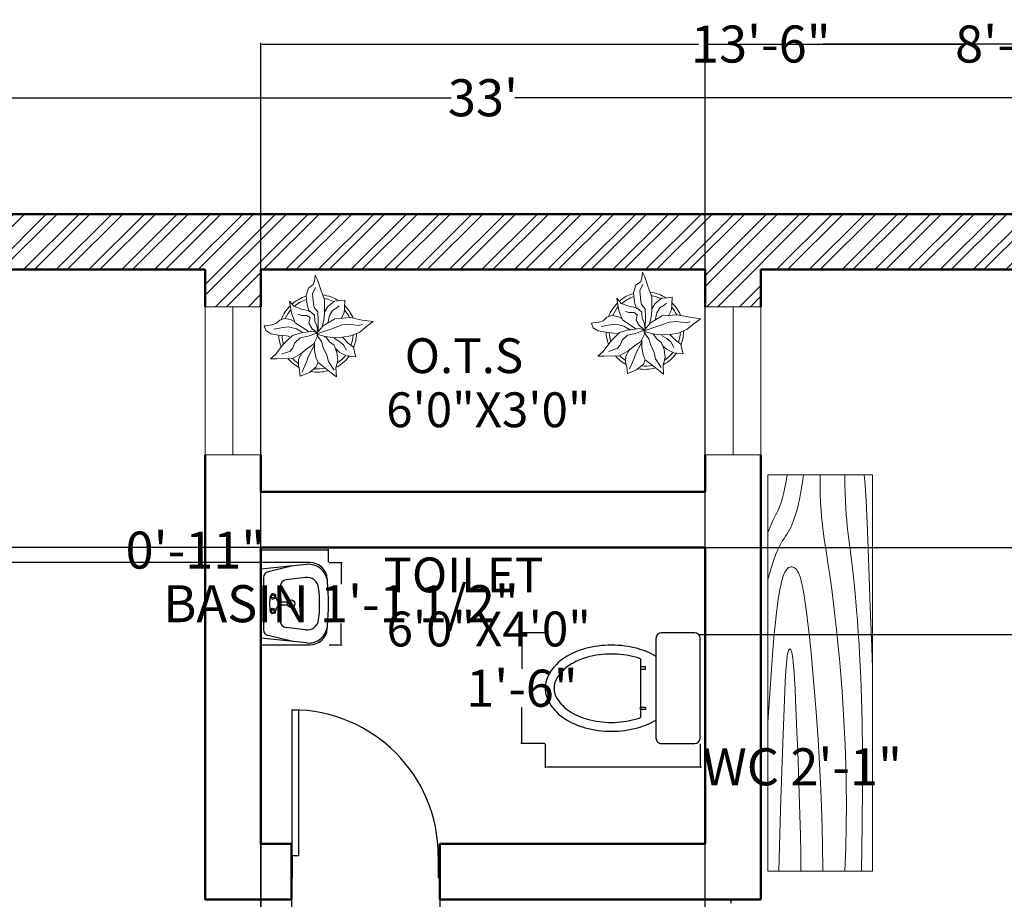
# Model space of a CAD drawing. Units: inches. Extents: x -71 to 434, y -519 to 67.
# Tile 6 of 7: x 110 to 270, y -80 to 62. Entities that reach past the tile are written whole.
import ezdxf

# ---------------------------------------------------------------- set-up
doc = ezdxf.new("R2010")
doc.units = ezdxf.units.IN
doc.header["$MEASUREMENT"] = 0
for name, color, linetype, lineweight in [('A-ANNO-DIMS', 7, 'Continuous', 18), ('A-AREA-IDEN', 7, 'Continuous', 25), ('A-FLOR-FIXT', 9, 'Continuous', 18), ('A-WALL-PATT', 8, 'Continuous', 13), ('CAY', 94, 'Continuous', 13), ('DOOR', 3, 'Continuous', 25), ('FURNITURE', 5, 'Continuous', 18), ('WALL', 50, 'Continuous', 50), ('WINDOW', 1, 'Continuous', 18)]:
    doc.layers.add(name, color=color, linetype=linetype, lineweight=lineweight)
doc.layers.add('THIET-BI', color=21, linetype='Continuous')
doc.styles.add('ATT', font='romans.shx')
doc.styles.get("Standard").update_dxf_attribs({"font": 'arial.ttf'})
doc.dimstyles.get("Standard").update_dxf_attribs({"dimtxt": 6, "dimasz": 0.18, "dimexe": 0.18, "dimexo": 0.0625, "dimgap": 0.09, "dimtad": 0, "dimtih": 1, "dimtoh": 1, "dimdec": 0, "dimzin": 0, "dimdsep": 46, "dimlunit": 3, "dimtxsty": 'Standard', "dimcen": 0.09, "dimadec": 0, "dimazin": 0, "dimtfac": 1, "dimtdec": 0, "dimtofl": 0, "dimtmove": 0, "dimatfit": 3, "dimfxl": 1, "dimtolj": 1, "dimtzin": 0, "dimarcsym": 0})

# ---------------------------------------------------------------- blocks, each defined once
blk = doc.blocks.new('Hutch - 19 x 72 in.')
for p, q in [((0, -19), (0, 0)), ((0, 0), (71.999994, 0)), ((71.999994, 0), (71.999994, -19)), ((71.999994, -19), (0, -19))]:
    blk.add_line(p, q)
for points in [[(26.99999, 0), (32.30411, -0.35238), (36.66731, -0.66276), (40.20336, -0.93603), (43.02603, -1.17708), (45.2491, -1.39079), (46.98632, -1.58203), (48.35147, -1.7557), (49.45833, -1.91667), (50.40388, -2.06917), (51.21809, -2.21484), (51.91414, -2.35465), (52.5052, -2.48958), (53.00447, -2.6206), (53.42512, -2.7487), (53.78035, -2.87484), (54.08333, -3), (54.34537, -3.12516), (54.57031, -3.2513), (54.76008, -3.37939), (54.91666, -3.51042), (55.04198, -3.64534), (55.13801, -3.78516), (55.2067, -3.93083), (55.24999, -4.08333), (55.26904, -4.24316), (55.26171, -4.40885), (55.22509, -4.57845), (55.15624, -4.75), (55.05224, -4.92155), (54.91015, -5.09115), (54.72704, -5.25684), (54.49999, -5.41667), (54.22493, -5.56934), (53.89322, -5.71615), (53.49511, -5.85905), (53.02083, -6), (52.4606, -6.14095), (51.80468, -6.28385), (51.04329, -6.43066), (50.16666, -6.58333), (49.16007, -6.74381), (47.98892, -6.91406), (46.61368, -7.09603), (44.99478, -7.29167), (43.09268, -7.50293), (40.86783, -7.73177), (38.28067, -7.98014), (35.29166, -8.25), (31.87654, -8.54053), (28.07226, -8.83984), (23.93107, -9.1333), (19.5052, -9.40625), (14.84692, -9.64404), (10.00846, -9.83203), (5.04207, -9.95557), (0, -10)], [(52.99999, 0), (54.87133, -0.53955), (56.39257, -1.03516), (57.61205, -1.48975), (58.57812, -1.90625), (59.3391, -2.2876), (59.94335, -2.63672), (60.4392, -2.95654), (60.87499, -3.25), (61.29247, -3.52002), (61.70702, -3.76953), (62.12743, -4.00146), (62.56249, -4.21875), (63.02099, -4.42432), (63.51171, -4.62109), (64.04345, -4.81201), (64.62499, -5), (65.26489, -5.1875), (65.9707, -5.375), (66.74975, -5.5625), (67.60937, -5.75), (68.55688, -5.9375), (69.5996, -6.125), (70.744867, -6.3125), (71.999994, -6.5)], [(61.49999, 0), (62.35961, -0.35254), (63.08007, -0.66406), (63.68627, -0.94043), (64.20312, -1.1875), (64.65551, -1.41113), (65.06835, -1.61719), (65.46655, -1.81152), (65.87499, -2), (66.31762, -2.1875), (66.81445, -2.375), (67.38452, -2.5625), (68.04687, -2.75), (68.82055, -2.9375), (69.7246, -3.125), (70.77807, -3.3125), (71.999994, -3.5)], [(0, -2), (11.2006, -2.34123), (19.90169, -2.62044), (26.43969, -2.84595), (31.15103, -3.02604), (34.37214, -3.16903), (36.43945, -3.2832), (37.68936, -3.37687), (38.45833, -3.45833), (39.02937, -3.53459), (39.472, -3.60742), (39.80232, -3.67733), (40.03645, -3.74479), (40.1905, -3.8103), (40.28059, -3.87435), (40.32283, -3.93742), (40.33333, -4), (40.32405, -4.0625), (40.29036, -4.125), (40.22346, -4.1875), (40.11458, -4.25), (39.95491, -4.3125), (39.73567, -4.375), (39.44807, -4.4375), (39.08333, -4.5), (38.62491, -4.56282), (38.02538, -4.6276), (37.22957, -4.69629), (36.18228, -4.77083), (34.82836, -4.85319), (33.11262, -4.94531), (30.97989, -5.04915), (28.37499, -5.16667), (25.27416, -5.29818), (21.77929, -5.4375), (18.02368, -5.57682), (14.14062, -5.70833), (10.26342, -5.82422), (6.52539, -5.91667), (3.05981, -5.97786), (0, -6)], [(71.999994, -9.5), (70.071934, -9.51147), (68.38801, -9.54492), (66.91113, -9.59888), (65.60416, -9.67187), (64.43001, -9.76245), (63.35156, -9.86914), (62.3317, -9.99048), (61.33333, -10.125), (60.32128, -10.27157), (59.26822, -10.43034), (58.14876, -10.60181), (56.93749, -10.78646), (55.60904, -10.98478), (54.13801, -11.19726), (52.49902, -11.4244), (50.66666, -11.66667), (48.62239, -11.92358), (46.37499, -12.19075), (43.9401, -12.46281), (41.33333, -12.73437), (38.57031, -13.00008), (35.66666, -13.25456), (32.63801, -13.49243), (29.49999, -13.70833), (26.26367, -13.89689), (22.92187, -14.05273), (19.46289, -14.17049), (15.875, -14.24479), (12.14648, -14.27026), (8.26562, -14.24154), (4.2207, -14.15324), (0, -14)], [(0, -17), (8.37556, -17.14274), (15.58268, -17.20443), (21.74194, -17.19775), (26.97395, -17.13542), (31.39933, -17.03011), (35.13866, -16.89453), (38.31257, -16.74137), (41.04166, -16.58333), (43.4322, -16.43083), (45.5332, -16.28516), (47.37931, -16.14534), (49.0052, -16.01042), (50.44555, -15.87939), (51.73502, -15.7513), (52.90828, -15.62516), (53.99999, -15.5), (55.04044, -15.37508), (56.04231, -15.25065), (57.01391, -15.1272), (57.96353, -15.00521), (58.89949, -14.88517), (59.83007, -14.76758), (60.76358, -14.65291), (61.70833, -14.54167), (62.6752, -14.43465), (63.68554, -14.33398), (64.76326, -14.24211), (65.93229, -14.16146), (67.21655, -14.09448), (68.63997, -14.04362), (70.226475, -14.01131), (71.999994, -14)], [(36.99999, -19), (42.40038, -18.8125), (47.95312, -18.625), (53.43554, -18.4375), (58.62499, -18.25), (63.29882, -18.0625), (67.23437, -17.875), (70.208978, -17.6875), (71.999994, -17.5)]]:
    blk.add_lwpolyline(points)
blk = doc.blocks.new('A$C793314D9')
at = {"layer": 'THIET-BI'}
for p, q in [((0, 675), (0, 525)), ((475, 700), (25, 700)), ((500, 525), (500, 675)), ((25, 500), (475, 500)), ((163.6, 452.4), (153.8, 452.4)), ((153.8, 452.4), (153.8, 429.9)), ((163.6, 429.9), (163.6, 452.4)), ((336.2, 452.4), (345.9, 452.4)), ((336.2, 429.9), (336.2, 452.4)), ((345.9, 452.4), (345.9, 429.9)), ((117.1, 430), (382.9, 430)), ((153.8, 429.9), (163.6, 429.9)), ((345.9, 429.9), (336.2, 429.9))]:
    blk.add_line(p, q, dxfattribs=at)
for centre, radius, start, end in [((25, 675), 25, 90, 180), ((475, 675), 25, 0, 90), ((25, 525), 25, 180, 270), ((383.8, 333.9), 323.5, 149.0966, 164.9269), ((116.2, 333.9), 323.5, 15.0731, 30.9034), ((475, 525), 25, 270, 0), ((513.7, 298.9), 458.1, 164.9269, 180), ((513.7, 298.9), 418.1, 164.9269, 180), ((383.8, 333.9), 283.5, 160.176, 164.9269), ((116.2, 333.9), 283.5, 15.0731, 19.824), ((-13.7, 298.9), 418.1, 0, 15.0731), ((-13.7, 298.9), 458.1, 0, 15.0731), ((513.7, 298.9), 458.1, 180, 195.0731), ((513.7, 298.9), 418.1, 180, 195.0731), ((-13.7, 298.9), 418.1, 344.9269, 360), ((-13.7, 298.9), 458.1, 344.9269, 0), ((383.8, 263.9), 323.5, 195.0731, 213.0315), ((383.8, 263.9), 283.5, 195.0731, 213.0315), ((116.2, 263.9), 283.5, 326.9685, 344.9269), ((116.2, 263.9), 323.5, 326.9685, 344.9269), ((301.7, 210.5), 185.5, 213.0315, 237.5002), ((198.3, 210.5), 185.5, 302.4998, 326.9685), ((301.7, 210.5), 225.5, 213.0315, 237.5002), ((250, 129.3), 89.3, 237.5002, 270), ((250, 129.3), 89.3, 270, 302.4998), ((198.3, 210.5), 225.5, 302.4998, 326.9685), ((250, 129.3), 129.3, 237.5002, 270), ((250, 129.3), 129.3, 270, 302.4998)]:
    blk.add_arc(centre, radius, start, end, dxfattribs=at)
blk = doc.blocks.new('*U13')
for p, q in [((0, 0), (0, -6)), ((40, 0), (40, -6))]:
    blk.add_line(p, q)
blk.add_lwpolyline([(0, 0), (0, 40), (1.75, 40), (1.75, 0)], close=True)
blk.add_arc((0, 0), 40, 0, 90)
blk = doc.blocks.new('*D17')
at = {"layer": 'A-ANNO-DIMS', "color": 0, "lineweight": -2, "transparency": 16777216}
for p, q in [((-12.59, 30.9), (-12.59, 49.86)), ((-12.41, 49.68), (180.23, 49.68)), ((383.23, 49.68), (190.59, 49.68)), ((383.41, 30.9), (383.41, 49.86))]:
    blk.add_line(p, q, dxfattribs=at)
at = {"layer": 'A-ANNO-DIMS', "color": 0, "transparency": 16777216}
for points in [[(-12.41, 49.71), (-12.41, 49.65), (-12.59, 49.68)], [(383.23, 49.71), (383.23, 49.65), (383.41, 49.68)]]:
    blk.add_solid(points, dxfattribs=at)
at = {"layer": 'Defpoints', "color": 0, "transparency": 16777216}
for p in [(383.41, 49.68), (-12.59, 30.83), (383.41, 30.83)]:
    blk.add_point(p, dxfattribs=at)
at = {"layer": 'A-ANNO-DIMS', "color": 0, "transparency": 16777216, "insert": (185.41, 49.68), "char_height": 6, "attachment_point": 5}
blk.add_mtext("\\A1;33'", dxfattribs=at)
blk = doc.blocks.new('12PPLT12')
at = {"color": 0, "linetype": 'ByBlock'}
for p, q in [((-0.05, 0.632), (-0.034, 0.694)), ((-0.034, 0.694), (-0.032, 0.751)), ((-0.032, 0.751), (-0.002, 0.689)), ((-0.002, 0.689), (0.044, 0.559)), ((-0.148, 0.486), (-0.116, 0.583)), ((-0.116, 0.583), (-0.05, 0.632)), ((-0.064, 0.51), (-0.026, 0.591)), ((-0.05, 0.38), (-0.064, 0.51)), ((0.044, 0.559), (0.09, 0.432)), ((-0.349, 0.334), (-0.362, 0.415)), ((-0.362, 0.415), (-0.303, 0.35)), ((-0.132, 0.367), (-0.148, 0.486)), ((0.09, 0.432), (0.09, 0.339)), ((0.134, 0.347), (0.22, 0.415)), ((0.22, 0.415), (0.291, 0.421)), ((0.291, 0.421), (0.35, 0.429)), ((0.35, 0.429), (0.348, 0.331)), ((-0.332, 0.247), (-0.349, 0.334)), ((-0.303, 0.35), (-0.208, 0.312)), ((-0.208, 0.312), (-0.105, 0.29)), ((-0.108, 0.279), (-0.132, 0.367)), ((-0.105, 0.29), (-0.037, 0.236)), ((-0.043, 0.334), (-0.05, 0.38)), ((0.003, 0.279), (-0.043, 0.334)), ((0.009, 0.169), (0.003, 0.279)), ((0.09, 0.339), (0.09, 0.253)), ((0.093, 0.282), (0.134, 0.347)), ((0.193, 0.293), (0.155, 0.228)), ((0.25, 0.328), (0.193, 0.293)), ((0.28, 0.353), (0.25, 0.328)), ((0.342, 0.266), (0.304, 0.19)), ((0.348, 0.331), (0.342, 0.266)), ((-0.487, 0.171), (-0.536, 0.125)), ((-0.425, 0.193), (-0.487, 0.171)), ((-0.346, 0.179), (-0.425, 0.193)), ((-0.292, 0.149), (-0.346, 0.179)), ((-0.289, 0.136), (-0.332, 0.247)), ((-0.194, 0.074), (-0.289, 0.136)), ((-0.205, 0.231), (-0.251, 0.247)), ((-0.137, 0.231), (-0.205, 0.231)), ((-0.097, 0.204), (-0.137, 0.231)), ((-0.11, 0.133), (-0.097, 0.204)), ((-0.069, 0.06), (-0.11, 0.133)), ((-0.037, 0.236), (-0.034, 0.158)), ((-0.034, 0.158), (-0.007, 0.101)), ((0.006, 0.027), (0.009, 0.169)), ((0.082, 0.174), (0.061, 0.082)), ((0.074, 0.098), (0.223, 0.188)), ((0.09, 0.253), (0.082, 0.174)), ((0.155, 0.228), (0.131, 0.13)), ((0.223, 0.188), (0.421, 0.204)), ((0.421, 0.204), (0.573, 0.171)), ((0.573, 0.171), (0.716, 0.152)), ((0.716, 0.152), (0.613, 0.074)), ((-0.671, 0.098), (-0.687, 0.095)), ((-0.687, 0.095), (-0.666, 0.036)), ((-0.59, 0.109), (-0.671, 0.098)), ((-0.666, 0.036), (-0.601, -0.005)), ((-0.536, 0.125), (-0.59, 0.109)), ((-0.563, 0.052), (-0.441, 0.074)), ((-0.441, 0.074), (-0.373, 0.084)), ((-0.373, 0.084), (-0.27, 0.057)), ((-0.229, 0.003), (-0.324, -0.027)), ((-0.27, 0.057), (-0.186, 0.006)), ((-0.069, 0.027), (-0.229, 0.003)), ((-0.108, 0.019), (-0.194, 0.074)), ((-0.01, 0.003), (-0.121, -0.038)), ((-0.01, 0.014), (-0.069, 0.06)), ((-0.002, 0.006), (-0.069, 0.027)), ((-0.018, -0.008), (0.074, 0.098)), ((-0.01, -0.005), (0.169, 0.055)), ((0.003, 0.017), (-0.01, 0.014)), ((0.003, -0.029), (-0.01, 0.003)), ((-0.007, 0.101), (0.003, 0.017)), ((0.169, 0.055), (0.315, 0.109)), ((0.315, 0.109), (0.413, 0.117)), ((0.413, 0.117), (0.524, 0.101)), ((0.545, 0.017), (0.429, -0.032)), ((0.524, 0.101), (0.578, 0.114)), ((0.613, 0.074), (0.545, 0.017)), ((-0.601, -0.005), (-0.503, -0.021)), ((-0.503, -0.021), (-0.4, -0.032)), ((-0.395, -0.094), (-0.452, -0.152)), ((-0.4, -0.032), (-0.357, -0.04)), ((-0.324, -0.027), (-0.395, -0.094)), ((-0.292, -0.122), (-0.316, -0.187)), ((-0.224, -0.059), (-0.292, -0.122)), ((-0.121, -0.038), (-0.224, -0.059)), ((-0.053, -0.14), (0.003, -0.029)), ((-0.037, -0.122), (-0.04, -0.219)), ((0.082, -0.038), (-0.018, -0.008)), ((-0.007, -0.024), (0.05, -0.105)), ((0.05, -0.105), (0.071, -0.181)), ((0.188, -0.054), (0.082, -0.038)), ((0.112, -0.051), (0.09, -0.043)), ((0.155, -0.108), (0.112, -0.051)), ((0.212, -0.152), (0.155, -0.108)), ((0.323, -0.051), (0.188, -0.054)), ((0.215, -0.062), (0.282, -0.103)), ((0.282, -0.103), (0.334, -0.146)), ((0.429, -0.032), (0.323, -0.051)), ((0.396, -0.124), (0.326, -0.054)), ((0.464, -0.176), (0.396, -0.124)), ((-0.452, -0.152), (-0.536, -0.268)), ((-0.387, -0.241), (-0.465, -0.268)), ((-0.352, -0.227), (-0.387, -0.241)), ((-0.316, -0.187), (-0.352, -0.227)), ((-0.193, -0.236), (-0.244, -0.33)), ((-0.213, -0.263), (-0.135, -0.195)), ((-0.135, -0.195), (-0.053, -0.14)), ((-0.119, -0.304), (-0.04, -0.148)), ((-0.04, -0.219), (-0.021, -0.308)), ((0.071, -0.181), (0.12, -0.282)), ((0.247, -0.246), (0.212, -0.152)), ((0.234, -0.2), (0.277, -0.241)), ((0.261, -0.349), (0.247, -0.246)), ((0.277, -0.241), (0.372, -0.287)), ((0.334, -0.146), (0.372, -0.217)), ((0.48, -0.257), (0.464, -0.176)), ((-0.536, -0.268), (-0.606, -0.328)), ((-0.606, -0.328), (-0.522, -0.328)), ((-0.522, -0.328), (-0.324, -0.325)), ((-0.324, -0.325), (-0.213, -0.263)), ((-0.244, -0.33), (-0.247, -0.406)), ((-0.199, -0.494), (-0.139, -0.358)), ((-0.139, -0.358), (-0.119, -0.304)), ((-0.021, -0.308), (0.006, -0.376)), ((-0.017, -0.432), (0.003, -0.378)), ((0.006, -0.376), (0.074, -0.428)), ((0.12, -0.282), (0.139, -0.363)), ((0.139, -0.363), (0.212, -0.474)), ((0.236, -0.444), (0.261, -0.349)), ((0.372, -0.287), (0.494, -0.301)), ((0.494, -0.301), (0.48, -0.257)), ((-0.247, -0.406), (-0.233, -0.471)), ((-0.233, -0.471), (-0.222, -0.551)), ((-0.148, -0.522), (-0.102, -0.503)), ((-0.102, -0.503), (-0.017, -0.432)), ((0.074, -0.428), (0.158, -0.496)), ((0.158, -0.496), (0.242, -0.561)), ((0.242, -0.561), (0.236, -0.444)), ((-0.222, -0.551), (-0.148, -0.522))]:
    blk.add_line(p, q, dxfattribs=at)
for radius, start, end in [(0.5, 107.123, 130.9816), (0.458, 107.9864, 130.5771), (0.5, 56.9563, 82.295), (0.458, 62.6899, 79.5345), (0.5, 134.8021, 159.1804), (0.458, 138.4756, 155.3347), (0.458, 26.2761, 41.1349), (0.5, 22.9768, 45.8473), (0.5, 182.503, 200.4563), (0.458, 183.2699, 197.4002), (0.458, 340.6559, 357.5057), (0.5, 338.5862, 359.7442), (0.5, 220.6606, 241.3393), (0.458, 225.0835, 237.5023), (0.5, 298.3455, 324.4541), (0.458, 303.3868, 322.0756), (0.5, 259.7038, 286.1281), (0.458, 264.1886, 282.4028)]:
    blk.add_arc((0, 0), radius, start, end, dxfattribs=at)
at = {"color": 0, "linetype": 'ByBlock', "style": 'ATT'}
for tag, p, flags in [('ITEM', (-1, -3.25), 3), ('ROOM_NUMBER', (-1, -4.583), 1)]:
    blk.add_attdef(tag, p, '', height=1, dxfattribs=dict(at, flags=flags))
blk = doc.blocks.new('TAM')
for p, q in [((-68.4, 12), (-49.4, 25.8)), ((-61.2, -10.4), (-68.4, 12)), ((-59.4, 6.8), (-61.2, 6.8)), ((-49.4, 25.8), (-30.4, 12)), ((-30.4, 12), (-37.6, -10.4)), ((50.6, 25.8), (31.6, 12)), ((31.6, 12), (38.8, -10.4)), ((69.6, 12), (50.6, 25.8)), ((60.6, 6.8), (62.4, 6.8)), ((62.4, -10.4), (69.6, 12)), ((-59.4, -10.4), (-49.4, -10.4)), ((-9.4, -60.4), (-9.4, -50.4)), ((-9.4, -90.4), (-9.4, -60.4)), ((10.6, -60.4), (10.6, -50.4)), ((10.6, -90.4), (10.6, -60.4)), ((62.4, -10.4), (50.6, -10.4)), ((-9.4, -90.4), (10.6, -90.4))]:
    blk.add_line(p, q)
for centre in [(-49.8, 6.8), (51, 6.8)]:
    blk.add_circle(centre, 10.4)
for centre, radius, start, end in [((0.6, -221.7), 252.5, 78.57881, 101.42119), ((-49.4, -50.4), 40, 0, 90), ((50.6, -50.4), 40, 90, 180)]:
    blk.add_arc(centre, radius, start, end)
blk = doc.blocks.new('A$C0E2F1A29')
at = {"layer": 'THIET-BI'}
for p, q in [((0, 460), (0, 126.9)), ((560, 460), (0, 460)), ((13, 148.3), (44.6, 460)), ((22.6, 242.8), (63.6, 409.5)), ((457.6, 440), (102.4, 440)), ((537.4, 242.8), (496.4, 409.5)), ((547, 148.3), (515.4, 460)), ((560, 126.9), (560, 460)), ((101.6, 155.5), (117.4, 286)), ((167.1, 330), (280, 330)), ((392.9, 330), (280, 330)), ((458.4, 155.5), (442.6, 286))]:
    blk.add_line(p, q, dxfattribs=at)
blk.add_circle((280, 253.2), 25.4, dxfattribs=at)
for centre, radius, start, end in [((102.4, 400), 40, 90, 166.19533), ((457.6, 400), 40, 13.80467, 90), ((167.1, 280), 50, 90, 173.07801), ((392.9, 280), 50, 6.92199, 90), ((142.3, 135.2), 130, 174.2113, 265.70941), ((181, 145.9), 80, 173.07801, 263.17143), ((379, 145.9), 80, 276.82857, 6.92199), ((417.7, 135.2), 130, 274.29059, 5.7887), ((120, 126.9), 120, 180, 265.03849), ((440, 126.9), 120, 274.96151, 0), ((280, 1970), 1970, 265.70941, 274.29059), ((280, 972.5), 912.5, 263.17143, 276.82857)]:
    blk.add_arc(centre, radius, start, end, dxfattribs=at)
blk.add_blockref('TAM', (279.2, 369.4), dxfattribs=at)
blk = doc.blocks.new('*D30')
at = {"layer": 'A-ANNO-DIMS', "color": 0, "lineweight": -2, "transparency": 16777216}
for p, q in [((195.49, -55), (195.49, -58.88)), ((220.59, -55), (220.59, -58.88)), ((195.67, -58.7), (220.41, -58.7)), ((220.59, -58.7), (220.77, -58.7))]:
    blk.add_line(p, q, dxfattribs=at)
at = {"layer": 'A-ANNO-DIMS', "color": 0, "transparency": 16777216}
for points in [[(195.67, -58.67), (195.67, -58.73), (195.49, -58.7)], [(220.41, -58.67), (220.41, -58.73), (220.59, -58.7)]]:
    blk.add_solid(points, dxfattribs=at)
at = {"layer": 'Defpoints', "color": 0, "transparency": 16777216}
for p in [(195.49, -54.93), (220.59, -54.93), (220.59, -58.7)]:
    blk.add_point(p, dxfattribs=at)
at = {"layer": 'A-ANNO-DIMS', "color": 0, "transparency": 16777216, "insert": (237.11, -58.7), "char_height": 6, "attachment_point": 5}
blk.add_mtext('\\A1;WC 2\'-1"', dxfattribs=at)
blk = doc.blocks.new('*D31')
at = {"layer": 'A-ANNO-DIMS', "color": 0, "lineweight": -2, "transparency": 16777216}
for p, q in [((195.42, -37), (191.54, -37)), ((191.72, -37.18), (191.72, -42.81)), ((191.72, -54.75), (191.72, -49.12)), ((195.42, -54.93), (191.54, -54.93))]:
    blk.add_line(p, q, dxfattribs=at)
at = {"layer": 'A-ANNO-DIMS', "color": 0, "transparency": 16777216}
for points in [[(191.69, -37.18), (191.75, -37.18), (191.72, -37)], [(191.69, -54.75), (191.75, -54.75), (191.72, -54.93)]]:
    blk.add_solid(points, dxfattribs=at)
at = {"layer": 'Defpoints', "color": 0, "transparency": 16777216}
for p in [(195.49, -37), (191.72, -54.93), (195.49, -54.93)]:
    blk.add_point(p, dxfattribs=at)
at = {"layer": 'A-ANNO-DIMS', "color": 0, "transparency": 16777216, "insert": (191.72, -45.97), "char_height": 6, "attachment_point": 5}
blk.add_mtext('\\A1;1\'-6"', dxfattribs=at)
blk = doc.blocks.new('*D36')
at = {"layer": 'A-ANNO-DIMS', "color": 0, "lineweight": -2, "transparency": 16777216}
for p, q in [((160.48, -25.61), (162.6, -25.61)), ((162.42, -25.79), (162.42, -29.09)), ((162.42, -38.77), (162.42, -35.47)), ((160.48, -38.95), (162.6, -38.95))]:
    blk.add_line(p, q, dxfattribs=at)
at = {"layer": 'A-ANNO-DIMS', "color": 0, "transparency": 16777216}
for points in [[(162.39, -25.79), (162.45, -25.79), (162.42, -25.61)], [(162.39, -38.77), (162.45, -38.77), (162.42, -38.95)]]:
    blk.add_solid(points, dxfattribs=at)
at = {"layer": 'Defpoints', "color": 0, "transparency": 16777216}
for p in [(160.41, -25.61), (162.42, -25.61), (160.41, -38.95)]:
    blk.add_point(p, dxfattribs=at)
at = {"layer": 'A-ANNO-DIMS', "color": 0, "transparency": 16777216, "insert": (162.42, -32.28), "char_height": 6, "attachment_point": 5}
blk.add_mtext('\\A1;BASIN 1\'-1 1/2"', dxfattribs=at)
blk = doc.blocks.new('*D37')
at = {"layer": 'A-ANNO-DIMS', "color": 0, "lineweight": -2, "transparency": 16777216}
for p, q in [((149.41, -23.6), (149.23, -23.6)), ((149.41, -25.54), (149.41, -23.42)), ((160.23, -23.6), (149.59, -23.6)), ((160.41, -25.54), (160.41, -23.42))]:
    blk.add_line(p, q, dxfattribs=at)
at = {"layer": 'A-ANNO-DIMS', "color": 0, "transparency": 16777216}
for points in [[(149.59, -23.57), (149.59, -23.63), (149.41, -23.6)], [(160.23, -23.57), (160.23, -23.63), (160.41, -23.6)]]:
    blk.add_solid(points, dxfattribs=at)
at = {"layer": 'Defpoints', "color": 0, "transparency": 16777216}
for p in [(149.41, -23.6), (149.41, -25.61), (160.41, -25.61)]:
    blk.add_point(p, dxfattribs=at)
at = {"layer": 'A-ANNO-DIMS', "color": 0, "transparency": 16777216, "insert": (138.83, -23.6), "char_height": 6, "attachment_point": 5}
blk.add_mtext('\\A1;0\'-11"', dxfattribs=at)
blk = doc.blocks.new('*D49')
at = {"layer": 'A-ANNO-DIMS', "color": 0, "lineweight": -2, "transparency": 16777216}
for p, q in [((221.41, -473.1), (221.41, 58.56)), ((221.59, 58.38), (262.84, 58.38)), ((320.23, 58.38), (278.98, 58.38)), ((320.41, -473.1), (320.41, 58.56))]:
    blk.add_line(p, q, dxfattribs=at)
at = {"layer": 'A-ANNO-DIMS', "color": 0, "transparency": 16777216}
for points in [[(221.59, 58.41), (221.59, 58.35), (221.41, 58.38)], [(320.23, 58.41), (320.23, 58.35), (320.41, 58.38)]]:
    blk.add_solid(points, dxfattribs=at)
at = {"layer": 'Defpoints', "color": 0, "transparency": 16777216}
for p in [(320.41, 58.38), (221.41, -473.17), (320.41, -473.17)]:
    blk.add_point(p, dxfattribs=at)
at = {"layer": 'A-ANNO-DIMS', "color": 0, "transparency": 16777216, "insert": (270.91, 58.38), "char_height": 6, "attachment_point": 5}
blk.add_mtext('\\A1;8\'-3"', dxfattribs=at)
blk = doc.blocks.new('*D56')
at = {"layer": 'A-ANNO-DIMS', "color": 0, "lineweight": -2, "transparency": 16777216}
for p, q in [((154.41, -71.23), (154.41, -509.9)), ((178.41, -71.23), (178.41, -509.9)), ((154.59, -509.72), (158.29, -509.72)), ((178.23, -509.72), (174.52, -509.72))]:
    blk.add_line(p, q, dxfattribs=at)
at = {"layer": 'A-ANNO-DIMS', "color": 0, "transparency": 16777216}
for points in [[(154.59, -509.69), (154.59, -509.75), (154.41, -509.72)], [(178.23, -509.69), (178.23, -509.75), (178.41, -509.72)]]:
    blk.add_solid(points, dxfattribs=at)
at = {"layer": 'Defpoints', "color": 0, "transparency": 16777216}
for p in [(154.41, -71.17), (178.41, -71.17), (178.41, -509.72)]:
    blk.add_point(p, dxfattribs=at)
at = {"layer": 'A-ANNO-DIMS', "color": 0, "transparency": 16777216, "insert": (166.41, -509.72), "char_height": 6, "attachment_point": 5}
blk.add_mtext('\\A1;2\'-0"', dxfattribs=at)
blk = doc.blocks.new('*D60')
at = {"layer": 'A-ANNO-DIMS', "color": 0, "lineweight": -2, "transparency": 16777216}
for p, q in [((149.35, -23.17), (-40.32, -23.17)), ((-40.14, -23.35), (-40.14, -25.43)), ((149.35, -25.61), (-40.32, -25.61)), ((-40.14, -25.79), (-40.32, -25.79)), ((-40.14, -25.61), (-40.14, -25.79))]:
    blk.add_line(p, q, dxfattribs=at)
at = {"layer": 'A-ANNO-DIMS', "color": 0, "transparency": 16777216}
for points in [[(-40.17, -23.35), (-40.11, -23.35), (-40.14, -23.17)], [(-40.17, -25.43), (-40.11, -25.43), (-40.14, -25.61)]]:
    blk.add_solid(points, dxfattribs=at)
at = {"layer": 'Defpoints', "color": 0, "transparency": 16777216}
for p in [(149.41, -23.17), (-40.14, -25.61), (149.41, -25.61)]:
    blk.add_point(p, dxfattribs=at)
at = {"layer": 'A-ANNO-DIMS', "color": 0, "transparency": 16777216, "insert": (-55.38, -25.79), "char_height": 6, "attachment_point": 5}
blk.add_mtext('\\A1;0\'-2 1/2"', dxfattribs=at)
blk = doc.blocks.new('*D61')
at = {"layer": 'A-ANNO-DIMS', "color": 0, "lineweight": -2, "transparency": 16777216}
for p, q in [((221.47, -23.17), (411.14, -23.17)), ((410.96, -23.35), (410.96, -27.11)), ((410.96, -37.08), (410.96, -33.32)), ((220.39, -37.26), (411.14, -37.26))]:
    blk.add_line(p, q, dxfattribs=at)
at = {"layer": 'A-ANNO-DIMS', "color": 0, "transparency": 16777216}
for points in [[(410.93, -23.35), (410.99, -23.35), (410.96, -23.17)], [(410.93, -37.08), (410.99, -37.08), (410.96, -37.26)]]:
    blk.add_solid(points, dxfattribs=at)
at = {"layer": 'Defpoints', "color": 0, "transparency": 16777216}
for p in [(221.41, -23.17), (220.33, -37.26), (410.96, -37.26)]:
    blk.add_point(p, dxfattribs=at)
at = {"layer": 'A-ANNO-DIMS', "color": 0, "transparency": 16777216, "insert": (410.96, -30.21), "char_height": 6, "attachment_point": 5}
blk.add_mtext('\\A1;1\'-2"', dxfattribs=at)
blk = doc.blocks.new('*D62')
at = {"layer": 'A-ANNO-DIMS', "color": 0, "lineweight": -2, "transparency": 16777216}
for p, q in [((149.41, -71.23), (149.41, -509.9)), ((154.41, -71.23), (154.41, -509.9)), ((149.59, -509.72), (154.23, -509.72)), ((154.41, -509.72), (154.59, -509.72))]:
    blk.add_line(p, q, dxfattribs=at)
at = {"layer": 'A-ANNO-DIMS', "color": 0, "transparency": 16777216}
for points in [[(149.59, -509.69), (149.59, -509.75), (149.41, -509.72)], [(154.23, -509.69), (154.23, -509.75), (154.41, -509.72)]]:
    blk.add_solid(points, dxfattribs=at)
at = {"layer": 'Defpoints', "color": 0, "transparency": 16777216}
for p in [(149.41, -71.17), (154.41, -71.17), (154.41, -509.72)]:
    blk.add_point(p, dxfattribs=at)
at = {"layer": 'A-ANNO-DIMS', "color": 0, "transparency": 16777216, "insert": (162.65, -509.72), "char_height": 6, "attachment_point": 5}
blk.add_mtext('\\A1;0\'-5"', dxfattribs=at)
blk = doc.blocks.new('*D69')
at = {"layer": 'A-ANNO-DIMS', "color": 0, "lineweight": -2, "transparency": 16777216}
for p, q in [((149.41, -215.1), (149.41, 58.56)), ((149.59, 58.38), (220.29, 58.38)), ((311.23, 58.38), (240.52, 58.38)), ((311.41, -215.1), (311.41, 58.56))]:
    blk.add_line(p, q, dxfattribs=at)
at = {"layer": 'A-ANNO-DIMS', "color": 0, "transparency": 16777216}
for points in [[(149.59, 58.41), (149.59, 58.35), (149.41, 58.38)], [(311.23, 58.41), (311.23, 58.35), (311.41, 58.38)]]:
    blk.add_solid(points, dxfattribs=at)
at = {"layer": 'Defpoints', "color": 0, "transparency": 16777216}
for p in [(311.41, 58.38), (149.41, -215.17), (311.41, -215.17)]:
    blk.add_point(p, dxfattribs=at)
at = {"layer": 'A-ANNO-DIMS', "color": 0, "transparency": 16777216, "insert": (230.41, 58.38), "char_height": 6, "attachment_point": 5}
blk.add_mtext('\\A1;13\'-6"', dxfattribs=at)

msp = doc.modelspace()

# ---------------------------------------------------------------- hatches: boundary and pattern name
at = {"layer": 'A-WALL-PATT'}
h = msp.add_hatch(dxfattribs=at)
h.set_pattern_fill('ANSI32', color=256, scale=10)
h.set_pattern_definition([(45, (-213.138, 0), (-2.65165, 2.65165), []), (45, (-211.37, 0), (-2.65165, 2.65165), [])])
h.paths.add_polyline_path([(383.41, 30.83), (230.41, 30.83), (149.41, 30.83), (-12.59, 30.83), (-12.59, -20.17), (-3.59, -20.17), (-3.59, 21.83), (140.41, 21.83), (140.41, 15.83), (149.41, 15.83), (149.41, 21.83), (221.41, 21.83), (221.41, 15.83), (230.41, 15.83), (230.41, 21.83), (374.41, 21.83), (374.41, -110.17), (369.41, -110.17), (369.41, -119.17), (374.41, -119.17), (374.41, -215.17), (320.41, -215.17), (320.41, -119.17), (345.41, -119.17), (345.41, -110.17), (221.41, -110.17), (221.41, -119.17), (311.41, -119.17), (311.41, -215.17), (192.42, -215.17), (192.42, -224.17), (221.41, -224.17), (221.41, -228.23), (230.41, -228.23), (230.41, -224.17), (374.41, -224.17), (374.41, -368.17), (230.41, -368.17), (230.41, -266.34), (221.41, -266.34), (221.41, -368.17), (192.08, -368.17), (192.08, -377.17), (230.41, -377.17), (374.41, -377.17), (374.41, -473.17), (230.41, -473.17), (212.41, -473.17), (212.41, -482.17), (383.41, -482.17), (383.41, -377.17), (383.41, -224.17), (383.41, -119.17)])
h.paths.add_polyline_path([(149.41, -110.17), (-3.59, -110.17), (-3.59, -68.17), (-12.59, -68.17), (-12.59, -276.67), (-3.59, -276.67), (-3.59, -224.17), (154.41, -224.17), (154.41, -215.17), (149.41, -215.17), (149.41, -154.17), (140.41, -154.17), (140.41, -215.17), (-3.59, -215.17), (-3.59, -119.17), (19.82, -119.17), (140.41, -119.17), (140.41, -124.17), (149.41, -124.17)])
h.paths.add_polyline_path([(84.91, -368.17), (-3.59, -368.17), (-3.59, -324.67), (-12.59, -324.67), (-12.59, -377.17), (-12.59, -401.17), (-3.59, -401.17), (-3.59, -377.17), (84.91, -377.17)], flags=17)
h.paths.add_polyline_path([(1.41, -473.17), (-3.59, -473.17), (-3.59, -468.17), (-12.59, -468.17), (-12.59, -482.17), (1.41, -482.17)], flags=17)

# ---------------------------------------------------------------- linework, layer by layer
at = {"layer": 'DOOR'}
for p, q in [((154.51, -76.69), (154.41, -76.69)), ((178.18, -76.69), (178.41, -76.69)), ((149.41, -80.78), (149.41, -80.17)), ((225.58, -80.78), (225.58, -80.17))]:
    msp.add_line(p, q, dxfattribs=at)
at = {"layer": 'WALL'}
for p, q in [((-12.59, 30.83), (149.41, 30.83)), ((149.41, 30.83), (230.41, 30.83)), ((230.41, 30.83), (383.41, 30.83)), ((-3.59, 21.83), (140.41, 21.83)), ((140.41, 15.83), (140.41, 21.83)), ((149.41, 21.83), (221.41, 21.83)), ((149.41, 15.83), (149.41, 21.83)), ((221.41, 21.83), (221.41, 15.83)), ((230.41, 21.83), (230.41, 15.83)), ((230.41, 21.83), (374.41, 21.83)), ((140.41, -80.17), (140.41, -8.17)), ((149.41, -14.17), (149.41, -8.17)), ((221.41, -8.17), (221.41, -14.17)), ((230.41, -8.17), (230.41, -23.17)), ((149.41, -14.17), (221.41, -14.17)), ((149.41, -23.17), (221.41, -23.17)), ((149.41, -71.17), (149.41, -23.17)), ((221.41, -71.17), (221.41, -23.17)), ((230.41, -80.17), (230.41, -23.17)), ((149.41, -71.17), (154.41, -71.17)), ((154.41, -80.17), (154.41, -71.17)), ((178.41, -80.17), (178.41, -71.17)), ((178.41, -71.17), (221.41, -71.17)), ((140.41, -80.17), (154.41, -80.17)), ((178.41, -80.17), (230.41, -80.17))]:
    msp.add_line(p, q, dxfattribs=at)
at = {"layer": 'WINDOW'}
for p, q in [((144.91, -8.17), (144.91, 15.83)), ((221.41, 15.83), (230.41, 15.83)), ((221.41, -8.17), (221.41, 15.83)), ((225.91, -8.17), (225.91, 15.83)), ((230.41, -8.17), (230.41, 15.83)), ((221.41, -8.17), (230.41, -8.17))]:
    msp.add_line(p, q, dxfattribs=at)
msp.add_lwpolyline([(149.41, -8.17), (140.41, -8.17), (140.41, 15.83), (149.41, 15.83)], close=True, dxfattribs=at)

# ---------------------------------------------------------------- block references
at = {"layer": 'A-FLOR-FIXT'}
for name, p, xscale, yscale, zscale, rotation in [('A$C0E2F1A29', (160.37, -38.95), 0.0238320021352253, 0.0238320021352253, 0.0238320021352253, 90), ('A$C793314D9', (195.49, -37), 0.0358683223870911, 0.0358683223870911, 0.0358683223870911, 270)]:
    msp.add_blockref(name, p, dxfattribs=dict(at, xscale=xscale, yscale=yscale, zscale=zscale, rotation=rotation))
at = {"layer": 'CAY', "xscale": 12.58515090877727, "yscale": 12.58515090877727, "zscale": 12.58515090877727}
for p in [(158.61, 11.51), (211.62, 11.97)]:
    msp.add_blockref('12PPLT12', p, dxfattribs=at)
at = {"layer": 'DOOR', "xscale": 0.5915936042264672, "yscale": 0.5915936042264672, "zscale": 0.5915936042264672}
msp.add_blockref('*U13', (154.51, -73.14), dxfattribs=at)
at = {"layer": 'FURNITURE', "xscale": 0.8917373781469976, "yscale": 0.8917373781469976, "zscale": 0.8917373781469976, "rotation": 90}
msp.add_blockref('Hutch - 19 x 72 in.', (231.53, -75.61), dxfattribs=at)

# ---------------------------------------------------------------- texts
at = {"layer": 'A-AREA-IDEN'}
for s, p in [('O.T.S', (172.73, 5.07)), ('6\'0"X3\'0"', (169.73, -3.69)), ('TOILET', (169.29, -30.44)), ('6\'0"X4\'0"', (169.79, -39.2))]:
    msp.add_text(s, height=5.643, dxfattribs=at).set_placement(p)

# ---------------------------------------------------------------- dimensions: what is measured, and where the dimension line sits
at = {"layer": 'A-ANNO-DIMS'}
for base, p1, p2, override, picture, middle in [((311.41, 58.38), (149.41, -215.17), (311.41, -215.17), {"dimdec": 1, "dimlfac": 1, "dimrnd": 0, "dimzin": 1, "dimdsep": 46, "dimlunit": 4, "dimfrac": 2}, '*D69', (230.41, 58.38)), ((320.41, 58.38), (221.41, -473.17), (320.41, -473.17), {"dimdec": 1, "dimlfac": 1, "dimrnd": 0, "dimzin": 1, "dimdsep": 46, "dimlunit": 4, "dimfrac": 2}, '*D49', (270.91, 58.38)), ((383.41, 49.68), (-12.59, 30.83), (383.41, 30.83), {"dimclrd": 0, "dimclre": 0, "dimclrt": 0}, '*D17', (185.41, 49.68)), ((154.41, -509.72), (149.41, -71.17), (154.41, -71.17), {"dimdec": 1, "dimlfac": 1, "dimrnd": 0, "dimzin": 1, "dimdsep": 46, "dimlunit": 4, "dimfrac": 2}, '*D62', (162.65, -509.72)), ((178.41, -509.72), (154.41, -71.17), (178.41, -71.17), {"dimdec": 1, "dimlfac": 1, "dimrnd": 0, "dimzin": 1, "dimdsep": 46, "dimlunit": 4, "dimfrac": 2}, '*D56', (166.41, -509.72))]:
    dim = msp.add_linear_dim(base=base, p1=p1, p2=p2, dimstyle='Standard', override=override, dxfattribs=at)
    dim.commit()
    dim.dimension.update_dxf_attribs({"geometry": picture, "text_midpoint": middle})
for base, p1, p2, angle, picture, middle in [((-40.14, -25.61), (149.41, -23.17), (149.41, -25.61), 90, '*D60', (-55.38, -25.79)), ((149.41, -23.6), (160.41, -25.61), (149.41, -25.61), 180, '*D37', (138.83, -23.6)), ((410.96, -37.26), (221.41, -23.17), (220.33, -37.26), 90, '*D61', (410.96, -30.21)), ((191.72, -54.93), (195.49, -37), (195.49, -54.93), 270, '*D31', (191.72, -45.97))]:
    dim = msp.add_linear_dim(base=base, p1=p1, p2=p2, angle=angle, dimstyle='Standard', override={"dimdec": 1, "dimlfac": 1, "dimrnd": 0, "dimzin": 1, "dimdsep": 46, "dimlunit": 4, "dimfrac": 2}, dxfattribs=at)
    dim.commit()
    dim.dimension.update_dxf_attribs({"geometry": picture, "text_midpoint": middle})
dim = msp.add_linear_dim(base=(162.42, -25.61), p1=(160.41, -38.95), p2=(160.41, -25.61), angle=90, text='BASIN <>', dimstyle='Standard', override={"dimdec": 1, "dimlfac": 1, "dimrnd": 0, "dimzin": 1, "dimdsep": 46, "dimlunit": 4, "dimfrac": 2}, dxfattribs=at)
dim.commit()
dim.dimension.update_dxf_attribs({"geometry": '*D36', "text_midpoint": (162.42, -32.28)})
dim = msp.add_linear_dim(base=(220.59, -58.7), p1=(195.49, -54.93), p2=(220.59, -54.93), text='WC <>', dimstyle='Standard', override={"dimdec": 1, "dimlfac": 1, "dimrnd": 0, "dimzin": 1, "dimdsep": 46, "dimlunit": 4, "dimfrac": 2}, dxfattribs=at)
dim.commit()
dim.dimension.update_dxf_attribs({"geometry": '*D30', "text_midpoint": (237.11, -58.7)})

doc.saveas('drawing.dxf')
